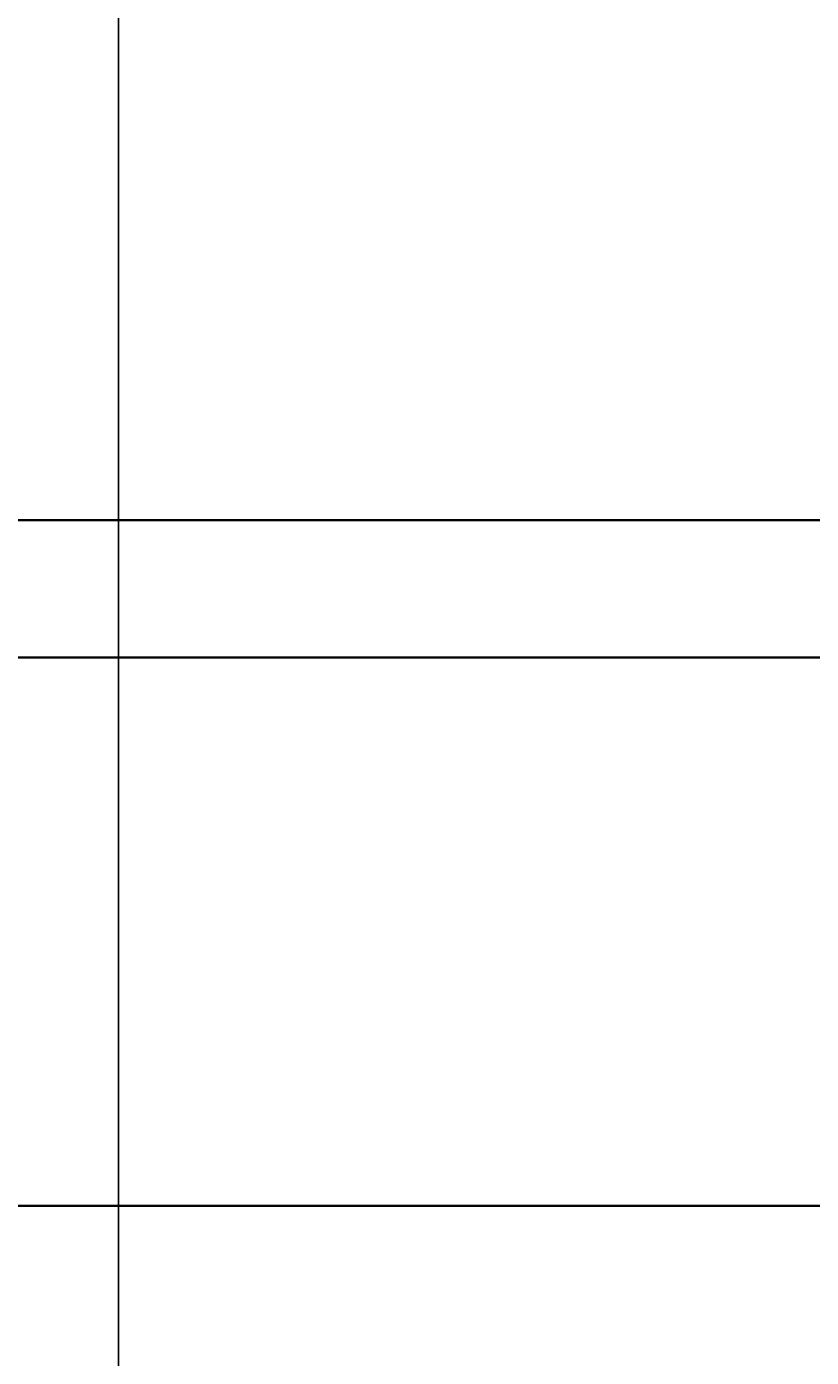
# Model space of a CAD drawing. Units: inches. Extents: x -6 to 289, y -8 to 323.
# Tile 53 of 107: x 169 to 186, y 124 to 153. Entities that reach past the tile are written whole.
import ezdxf

# ---------------------------------------------------------------- set-up
doc = ezdxf.new("R2010")
doc.units = ezdxf.units.IN
doc.header["$MEASUREMENT"] = 0
doc.layers.add('A-ANNO-DIMS', color=2, linetype='Continuous', lineweight=18)
doc.layers.add('A-ELEV', color=7, linetype='Continuous', lineweight=35)
doc.styles.get("Standard").update_dxf_attribs({"font": 'arial.ttf'})
doc.dimstyles.get("Standard").update_dxf_attribs({"dimtxt": 0.18, "dimasz": 0.18, "dimexe": 0.18, "dimexo": 0.0625, "dimgap": 0.09, "dimtad": 0, "dimtih": 1, "dimtoh": 1, "dimdec": 4, "dimzin": 0, "dimdsep": 46, "dimtxsty": 'Standard', "dimcen": 0.09, "dimadec": 0, "dimazin": 0, "dimtfac": 1, "dimtdec": 4, "dimtofl": 0, "dimtmove": 0, "dimatfit": 3, "dimfxl": 1, "dimtolj": 1, "dimtzin": 0, "dimarcsym": 0})

# ---------------------------------------------------------------- blocks, each defined once
blk = doc.blocks.new('*D24')
at = {"layer": 'A-ANNO-DIMS', "color": 0, "lineweight": -2, "transparency": 16777216}
for p, q in [((126.946, 178.654), (288.653, 178.654)), ((288.473, 178.474), (288.473, 159.153)), ((288.473, 139.469), (288.473, 158.789)), ((259.226, 139.289), (288.653, 139.289))]:
    blk.add_line(p, q, dxfattribs=at)
at = {"layer": 'A-ANNO-DIMS', "color": 0, "transparency": 16777216}
for points in [[(288.443, 178.474), (288.503, 178.474), (288.473, 178.654)], [(288.443, 139.469), (288.503, 139.469), (288.473, 139.289)]]:
    blk.add_solid(points, dxfattribs=at)
at = {"layer": 'Defpoints', "color": 0, "transparency": 16777216}
for p in [(126.883, 178.654), (288.473, 178.654), (259.164, 139.289)]:
    blk.add_point(p, dxfattribs=at)
at = {"layer": 'A-ANNO-DIMS', "color": 0, "transparency": 16777216, "insert": (288.473, 158.971), "char_height": 0.18, "attachment_point": 5}
blk.add_mtext('\\A1;39.365', dxfattribs=at)
blk = doc.blocks.new('*D78')
at = {"layer": 'A-ANNO-DIMS', "color": 0, "lineweight": -2, "transparency": 16777216}
for p, q in [((168.296, 51.148), (168.296, 322.969)), ((171.296, 51.148), (171.296, 322.969)), ((168.476, 322.789), (169.647, 322.789)), ((171.116, 322.789), (169.945, 322.789))]:
    blk.add_line(p, q, dxfattribs=at)
at = {"layer": 'A-ANNO-DIMS', "color": 0, "transparency": 16777216}
for points in [[(168.476, 322.819), (168.476, 322.759), (168.296, 322.789)], [(171.116, 322.819), (171.116, 322.759), (171.296, 322.789)]]:
    blk.add_solid(points, dxfattribs=at)
at = {"layer": 'Defpoints', "color": 0, "transparency": 16777216}
for p in [(171.296, 322.789), (168.296, 51.085), (171.296, 51.085)]:
    blk.add_point(p, dxfattribs=at)
at = {"layer": 'A-ANNO-DIMS', "color": 0, "transparency": 16777216, "insert": (169.796, 322.789), "char_height": 0.18, "attachment_point": 5}
blk.add_mtext('\\A1;3', dxfattribs=at)
blk = doc.blocks.new('*D79')
at = {"layer": 'A-ANNO-DIMS', "color": 0, "lineweight": -2, "transparency": 16777216}
for p, q in [((171.296, 118.033), (171.296, 322.969)), ((188.292, 116.842), (188.292, 322.969)), ((171.476, 322.789), (179.339, 322.789)), ((188.112, 322.789), (180.249, 322.789))]:
    blk.add_line(p, q, dxfattribs=at)
at = {"layer": 'A-ANNO-DIMS', "color": 0, "transparency": 16777216}
for points in [[(171.476, 322.819), (171.476, 322.759), (171.296, 322.789)], [(188.112, 322.819), (188.112, 322.759), (188.292, 322.789)]]:
    blk.add_solid(points, dxfattribs=at)
at = {"layer": 'Defpoints', "color": 0, "transparency": 16777216}
for p in [(188.292, 322.789), (171.296, 117.971), (188.292, 116.779)]:
    blk.add_point(p, dxfattribs=at)
at = {"layer": 'A-ANNO-DIMS', "color": 0, "transparency": 16777216, "insert": (179.794, 322.789), "char_height": 0.18, "attachment_point": 5}
blk.add_mtext('\\A1;16.996', dxfattribs=at)

msp = doc.modelspace()

# ---------------------------------------------------------------- linework, layer by layer
at = {"layer": 'A-ELEV'}
for p, q in [((115.1638, 139.2888), (259.1638, 139.2888)), ((259.1638, 127.2888), (115.1638, 127.2888)), ((115.1638, 127.2888), (259.1638, 127.2888))]:
    msp.add_line(p, q, dxfattribs=at)
for points in [[(247.1638, 139.2888), (115.1638, 139.2888), (115.1638, 162.3484), (247.1638, 162.3484)], [(244.1638, 142.2888), (118.1638, 142.2888), (118.1638, 159.3484), (244.1638, 159.3484)]]:
    msp.add_lwpolyline(points, close=True, dxfattribs=at)

# ---------------------------------------------------------------- dimensions: what is measured, and where the dimension line sits
at = {"layer": 'A-ANNO-DIMS'}
for base, p1, p2, override, picture, middle in [((171.296, 322.7888), (168.296, 51.0851), (171.296, 51.0851), {"dimdec": 0, "dimlfac": 1, "dimrnd": 0, "dimzin": 0, "dimdsep": 46, "dimlunit": 2}, '*D78', (169.796, 322.7888)), ((188.2918, 322.7888), (171.296, 117.9706), (188.2918, 116.7795), {"dimdec": 3, "dimlfac": 1, "dimrnd": 0, "dimzin": 0, "dimdsep": 46, "dimlunit": 2}, '*D79', (179.7939, 322.7888))]:
    dim = msp.add_linear_dim(base=base, p1=p1, p2=p2, dimstyle='Standard', override=override, dxfattribs=at)
    dim.commit()
    dim.dimension.update_dxf_attribs({"geometry": picture, "text_midpoint": middle})
dim = msp.add_linear_dim(base=(288.4733, 178.654), p1=(259.1638, 139.2888), p2=(126.8835, 178.654), angle=90, dimstyle='Standard', override={"dimdec": 3, "dimlfac": 1, "dimrnd": 0, "dimzin": 0, "dimdsep": 46, "dimlunit": 2}, dxfattribs=at)
dim.commit()
dim.dimension.update_dxf_attribs({"geometry": '*D24', "text_midpoint": (288.4733, 158.9714)})

doc.saveas('drawing.dxf')
